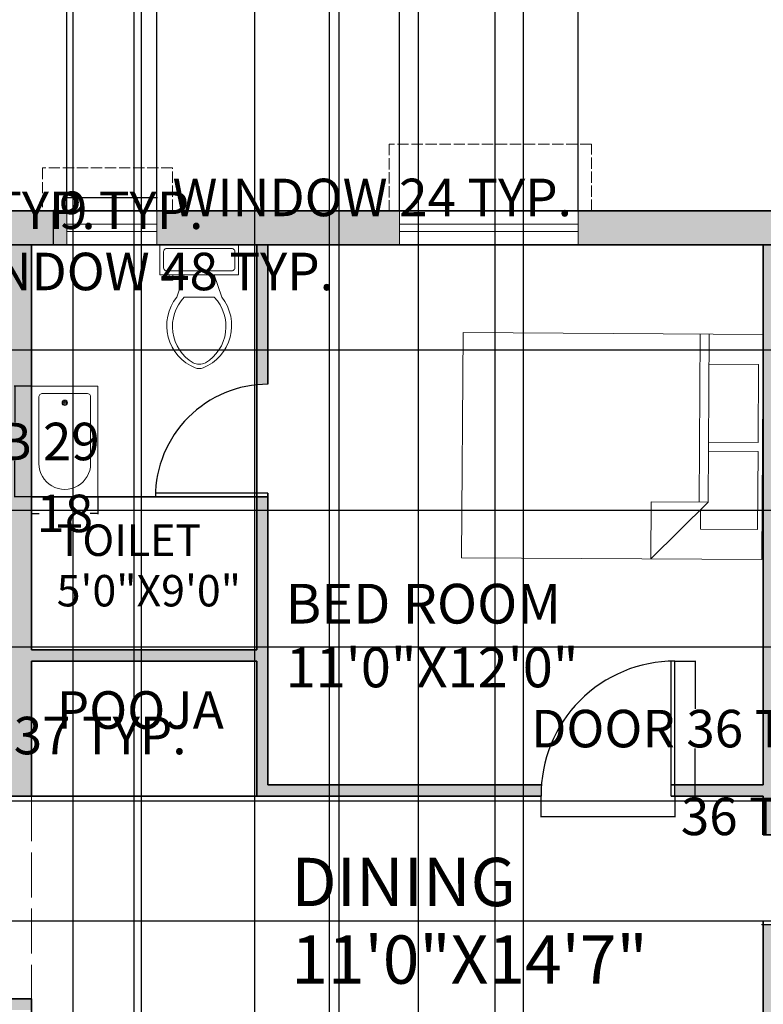
# Model space of a CAD drawing. Units: inches. Extents: x 300 to 1007, y 2 to 1069.
# Tile 5 of 12: x 568 to 766, y 271 to 533. Entities that reach past the tile are written whole.
import ezdxf

# ---------------------------------------------------------------- set-up
doc = ezdxf.new("R2010")
doc.units = ezdxf.units.IN
doc.header["$MEASUREMENT"] = 0
doc.linetypes.add('ACAD_ISO02W100', pattern=[15, 12, -3])
for name, color, linetype, lineweight in [('A-ANNO-DIMS', 2, 'Continuous', 18), ('A-AREA-IDEN', 7, 'Continuous', 18), ('A-DOOR', 3, 'Continuous', 25), ('A-FLOR-FIXT', 9, 'Continuous', 18), ('A-FURN', 8, 'Continuous', 18), ('A-GLAZ', 4, 'Continuous', 18), ('A-GLAZ-OVHD', 8, 'ACAD_ISO02W100', 13), ('A-WALL', 7, 'Continuous', 35), ('A-WALL-OVHD', 8, 'ACAD_ISO02W100', 18)]:
    doc.layers.add(name, color=color, linetype=linetype, lineweight=lineweight)
doc.layers.add('A-WALL-PATT', color=9, linetype='Continuous', lineweight=9, true_color=0xc7c8ca)
doc.styles.get("Standard").update_dxf_attribs({"font": 'arial.ttf'})
doc.dimstyles.get("Standard").update_dxf_attribs({"dimtxt": 10, "dimasz": 0.18, "dimexe": 0.18, "dimexo": 0.0625, "dimgap": 0.09, "dimtad": 0, "dimtih": 1, "dimtoh": 1, "dimdec": 0, "dimzin": 0, "dimdsep": 46, "dimlunit": 3, "dimtxsty": 'Standard', "dimcen": 0.09, "dimadec": 0, "dimazin": 0, "dimtfac": 1, "dimtdec": 0, "dimtofl": 0, "dimtmove": 0, "dimatfit": 3, "dimfxl": 1, "dimtolj": 1, "dimtzin": 0, "dimarcsym": 0})

# ---------------------------------------------------------------- blocks, each defined once
blk = doc.blocks.new('Bed - Queen')
for p, q in [((0, -80.00003), (0, 0)), ((0, 0), (59.99999, 0)), ((59.99999, 0), (59.99999, -80.00003)), ((7.99999, -1.2), (28.79998, -1.2)), ((7.99999, -14.4), (7.99999, -1.2)), ((28.79998, -1.2), (28.79998, -14.4)), ((31.19999, -1.2), (51.99999, -1.2)), ((31.19999, -14.4), (31.19999, -1.2)), ((51.99999, -1.2), (51.99999, -16.4)), ((0, -14.4), (44.8, -14.4)), ((59.99999, -29.6), (44.8, -14.4)), ((44.8, -14.4), (44.8, -29.6)), ((44.8, -16.8), (0, -16.8)), ((51.99999, -16.4), (46.79936, -16.4)), ((44.8, -29.6), (59.99999, -29.6)), ((59.99999, -80.00003), (0, -80.00003))]:
    blk.add_line(p, q)
blk = doc.blocks.new('Bath Tub - 26 x 60 in.')
for p, q in [((8, -18), (10, -18)), ((9, -17), (9, -19))]:
    blk.add_line(p, q)
blk.add_lwpolyline([(0, -36), (0, 0), (60, 0), (60, -36)], close=True)
for points in [[(6, -4), (42, -4)], [(4, -30), (4, -6)], [(42, -32), (6, -32)]]:
    blk.add_lwpolyline(points)
for radius in [1.5, 1]:
    blk.add_circle((9, -18), radius)
for centre, radius, start, end in [((5.75, -5.75), 1.77, 81.8699, 188.1301), ((42, -18), 14, 270, 90), ((5.75, -30.25), 1.77, 171.8699, 278.1301)]:
    blk.add_arc(centre, radius, start, end)
blk = doc.blocks.new('Toilet - top')
for p, q in [((9.5, -6), (9.5, -2)), ((-10, -8.5), (-8, -8.5)), ((-10, -9.5), (-10, -8.5)), ((-7, -9.5), (-10, -9.5)), ((-8, -8.5), (-8, -8)), ((-7, -8), (-7, -9.5)), ((-4, -8), (-6, -14)), ((4, -8), (6, -14)), ((4, -14), (-4, -14))]:
    blk.add_line(p, q)
blk.add_lwpolyline([(10.5, -8), (10.5, 0), (-10.5, 0), (-10.5, -8)], close=True)
for points in [[(-9.5, -2), (-9.5, -6)], [(8.5, -1), (-8.5, -1)], [(-8.5, -7), (8.5, -7)]]:
    blk.add_lwpolyline(points)
for centre, radius, start, end in [((-8.62, -1.88), 0.884, 81.8699, 188.1301), ((8.62, -1.88), 0.884, 351.8699, 98.1301), ((-8.62, -6.12), 0.884, 171.8699, 278.1301), ((8.62, -6.12), 0.884, 261.8699, 8.1301), ((3.52, -21.58), 12.17, 141.4691, 247.9714), ((4.2, -21.82), 11.33, 136.3677, 238.9468), ((-3.52, -21.58), 12.17, 292.0284, 38.5307), ((-4.2, -21.82), 11.33, 301.053, 43.6321), ((0, -27.88), 4, 245.7318, 294.2682), ((0, -29), 4, 254.8605, 285.1395)]:
    blk.add_arc(centre, radius, start, end)
blk = doc.blocks.new('WIN-47_5-8')
for p, q in [((-47.61, 0), (-47.61, 4.5)), ((-47.61, 4.5), (-47.61, -4.5)), ((0, -4.5), (0, 4.5)), ((0, 1), (-47.61, 1)), ((0, -1), (-47.61, -1))]:
    blk.add_line(p, q)
blk = doc.blocks.new('WIN-24')
for p, q in [((0, -4.5), (0, 4.5)), ((23.96, 0), (23.96, 4.5)), ((23.96, 4.5), (23.96, -4.5)), ((0, 1), (23.96, 1)), ((0, -1), (23.96, -1))]:
    blk.add_line(p, q)
blk = doc.blocks.new('WINDOW-HOOD-54')
at = {"ltscale": 0.25}
for p, q in [((0, 17.83), (-53.97, 17.83)), ((-53.97, 17.83), (-53.97, 0)), ((0, 0), (0, 17.83))]:
    blk.add_line(p, q, dxfattribs=at)
blk = doc.blocks.new('DOOR-SINGLE-30')
for p, q in [((0, 0), (30, 0)), ((0, -1), (0, 0)), ((0, -1), (30, -1))]:
    blk.add_line(p, q)
blk.add_arc((0, 0), 30, 270, 0)
blk = doc.blocks.new('DOOR-SINGLE-36')
for p, q in [((-1, 0), (-1, 36)), ((0, 0), (0, 36))]:
    blk.add_line(p, q)
blk.add_arc((0, 0.34), 35.66, 90, 180.5503)
blk = doc.blocks.new('*D35')
at = {"layer": 'A-ANNO-DIMS', "color": 0, "lineweight": -2, "transparency": 16777216}
for p, q in [((571.06, 435.66), (566.52, 435.66)), ((566.7, 435.48), (566.7, 426.11)), ((566.7, 406.35), (566.7, 415.72)), ((571.06, 406.17), (566.52, 406.17))]:
    blk.add_line(p, q, dxfattribs=at)
at = {"layer": 'A-ANNO-DIMS', "color": 0, "transparency": 16777216}
for points in [[(566.67, 435.48), (566.73, 435.48), (566.7, 435.66)], [(566.67, 406.35), (566.73, 406.35), (566.7, 406.17)]]:
    blk.add_solid(points, dxfattribs=at)
at = {"layer": 'Defpoints', "color": 0, "transparency": 16777216}
for p in [(571.12, 435.66), (566.7, 406.17), (571.12, 406.17)]:
    blk.add_point(p, dxfattribs=at)
at = {"layer": 'A-ANNO-DIMS', "color": 0, "transparency": 16777216, "insert": (566.7, 420.92), "char_height": 10, "attachment_point": 5}
blk.add_mtext('\\A1;TUB 29', dxfattribs=at)
blk = doc.blocks.new('*D36')
at = {"layer": 'A-ANNO-DIMS', "color": 0, "lineweight": -2, "transparency": 16777216}
for p, q in [((571.12, 406.11), (571.12, 401.57)), ((588.81, 406.11), (588.81, 401.57)), ((571.3, 401.75), (573.18, 401.75)), ((588.63, 401.75), (586.76, 401.75))]:
    blk.add_line(p, q, dxfattribs=at)
at = {"layer": 'A-ANNO-DIMS', "color": 0, "transparency": 16777216}
for points in [[(571.3, 401.78), (571.3, 401.72), (571.12, 401.75)], [(588.63, 401.78), (588.63, 401.72), (588.81, 401.75)]]:
    blk.add_solid(points, dxfattribs=at)
at = {"layer": 'Defpoints', "color": 0, "transparency": 16777216}
for p in [(571.12, 406.17), (588.81, 406.17), (588.81, 401.75)]:
    blk.add_point(p, dxfattribs=at)
at = {"layer": 'A-ANNO-DIMS', "color": 0, "transparency": 16777216, "insert": (579.97, 401.75), "char_height": 10, "attachment_point": 5}
blk.add_mtext('\\A1;18', dxfattribs=at)
blk = doc.blocks.new('*D52')
at = {"layer": 'A-ANNO-DIMS', "color": 0, "lineweight": -2, "transparency": 16777216}
for p, q in [((528.12, 355.06), (528.12, 342.35)), ((564.79, 355.06), (564.79, 342.35)), ((528.3, 342.53), (564.61, 342.53)), ((564.79, 342.53), (564.97, 342.53))]:
    blk.add_line(p, q, dxfattribs=at)
at = {"layer": 'A-ANNO-DIMS', "color": 0, "transparency": 16777216}
for points in [[(528.3, 342.56), (528.3, 342.5), (528.12, 342.53)], [(564.61, 342.56), (564.61, 342.5), (564.79, 342.53)]]:
    blk.add_solid(points, dxfattribs=at)
at = {"layer": 'Defpoints', "color": 0, "transparency": 16777216}
for p in [(528.12, 355.13), (564.79, 355.13), (564.79, 342.53)]:
    blk.add_point(p, dxfattribs=at)
at = {"layer": 'A-ANNO-DIMS', "color": 0, "transparency": 16777216, "insert": (589.39, 342.53), "char_height": 10, "attachment_point": 5}
blk.add_mtext('\\A1;37 TYP.', dxfattribs=at)
blk = doc.blocks.new('*D55')
at = {"layer": 'A-ANNO-DIMS', "color": 0, "lineweight": -2, "transparency": 16777216}
for p, q in [((493.48, 473.32), (493.48, 466.06)), ((541.08, 473.32), (541.08, 466.06)), ((493.66, 466.24), (540.9, 466.24)), ((541.08, 466.24), (541.26, 466.24))]:
    blk.add_line(p, q, dxfattribs=at)
at = {"layer": 'A-ANNO-DIMS', "color": 0, "transparency": 16777216}
for points in [[(493.66, 466.27), (493.66, 466.21), (493.48, 466.24)], [(540.9, 466.27), (540.9, 466.21), (541.08, 466.24)]]:
    blk.add_solid(points, dxfattribs=at)
at = {"layer": 'Defpoints', "color": 0, "transparency": 16777216}
for p in [(493.48, 473.38), (541.08, 473.38), (541.08, 466.24)]:
    blk.add_point(p, dxfattribs=at)
at = {"layer": 'A-ANNO-DIMS', "color": 0, "transparency": 16777216, "insert": (598.48, 466.24), "char_height": 10, "attachment_point": 5}
blk.add_mtext('\\A1;WINDOW 48 TYP.', dxfattribs=at)
blk = doc.blocks.new('*D56')
at = {"layer": 'A-ANNO-DIMS', "color": 0, "lineweight": -2, "transparency": 16777216}
for p, q in [((541.14, 482.38), (548.4, 482.38)), ((548.22, 482.38), (548.22, 482.56)), ((548.22, 482.56), (548.4, 482.56)), ((548.22, 473.56), (548.22, 482.2)), ((541.14, 473.38), (548.4, 473.38))]:
    blk.add_line(p, q, dxfattribs=at)
at = {"layer": 'A-ANNO-DIMS', "color": 0, "transparency": 16777216}
for points in [[(548.19, 482.2), (548.25, 482.2), (548.22, 482.38)], [(548.19, 473.56), (548.25, 473.56), (548.22, 473.38)]]:
    blk.add_solid(points, dxfattribs=at)
at = {"layer": 'Defpoints', "color": 0, "transparency": 16777216}
for p in [(541.08, 482.38), (548.22, 482.38), (541.08, 473.38)]:
    blk.add_point(p, dxfattribs=at)
at = {"layer": 'A-ANNO-DIMS', "color": 0, "transparency": 16777216, "insert": (568.95, 482.56), "char_height": 10, "attachment_point": 5}
blk.add_mtext('\\A1;9 TYP.', dxfattribs=at)
blk = doc.blocks.new('*D57')
at = {"layer": 'A-ANNO-DIMS', "color": 0, "lineweight": -2, "transparency": 16777216}
for p, q in [((580.53, 482.45), (580.53, 486.16)), ((580.71, 485.98), (604.31, 485.98)), ((604.49, 482.45), (604.49, 486.16)), ((604.49, 485.98), (604.67, 485.98))]:
    blk.add_line(p, q, dxfattribs=at)
at = {"layer": 'A-ANNO-DIMS', "color": 0, "transparency": 16777216}
for points in [[(580.71, 486.01), (580.71, 485.95), (580.53, 485.98)], [(604.31, 486.01), (604.31, 485.95), (604.49, 485.98)]]:
    blk.add_solid(points, dxfattribs=at)
at = {"layer": 'Defpoints', "color": 0, "transparency": 16777216}
for p in [(604.49, 485.98), (580.53, 482.38), (604.49, 482.38)]:
    blk.add_point(p, dxfattribs=at)
at = {"layer": 'A-ANNO-DIMS', "color": 0, "transparency": 16777216, "insert": (661.89, 485.98), "char_height": 10, "attachment_point": 5}
blk.add_mtext('\\A1;WINDOW 24 TYP.', dxfattribs=at)
blk = doc.blocks.new('*D58')
at = {"layer": 'A-ANNO-DIMS', "color": 0, "lineweight": -2, "transparency": 16777216}
for p, q in [((580.47, 482.38), (576.76, 482.38)), ((576.94, 482.38), (576.94, 482.56)), ((576.94, 482.56), (577.12, 482.56)), ((576.94, 473.56), (576.94, 482.2)), ((580.47, 473.38), (576.76, 473.38))]:
    blk.add_line(p, q, dxfattribs=at)
at = {"layer": 'A-ANNO-DIMS', "color": 0, "transparency": 16777216}
for points in [[(576.91, 482.2), (576.97, 482.2), (576.94, 482.38)], [(576.91, 473.56), (576.97, 473.56), (576.94, 473.38)]]:
    blk.add_solid(points, dxfattribs=at)
at = {"layer": 'Defpoints', "color": 0, "transparency": 16777216}
for p in [(576.94, 482.38), (580.53, 482.38), (580.53, 473.38)]:
    blk.add_point(p, dxfattribs=at)
at = {"layer": 'A-ANNO-DIMS', "color": 0, "transparency": 16777216, "insert": (597.66, 482.56), "char_height": 10, "attachment_point": 5}
blk.add_mtext('\\A1;9 TYP.', dxfattribs=at)
blk = doc.blocks.new('*D65')
at = {"layer": 'A-ANNO-DIMS', "color": 0, "lineweight": -2, "transparency": 16777216}
for p, q in [((742.62, 362.38), (748.14, 362.38)), ((747.96, 362.2), (747.96, 349.65)), ((747.96, 326.56), (747.96, 339.12)), ((742.62, 326.38), (748.14, 326.38))]:
    blk.add_line(p, q, dxfattribs=at)
at = {"layer": 'A-ANNO-DIMS', "color": 0, "transparency": 16777216}
for points in [[(747.93, 362.2), (747.99, 362.2), (747.96, 362.38)], [(747.93, 326.56), (747.99, 326.56), (747.96, 326.38)]]:
    blk.add_solid(points, dxfattribs=at)
at = {"layer": 'Defpoints', "color": 0, "transparency": 16777216}
for p in [(742.56, 362.38), (747.96, 362.38), (742.56, 326.38)]:
    blk.add_point(p, dxfattribs=at)
at = {"layer": 'A-ANNO-DIMS', "color": 0, "transparency": 16777216, "insert": (747.96, 344.38), "char_height": 10, "attachment_point": 5}
blk.add_mtext('\\A1;DOOR 36 TYP.', dxfattribs=at)
blk = doc.blocks.new('*D66')
at = {"layer": 'A-ANNO-DIMS', "color": 0, "lineweight": -2, "transparency": 16777216}
for p, q in [((706.81, 326.32), (706.81, 320.8)), ((742.56, 326.32), (742.56, 320.8)), ((706.99, 320.98), (742.38, 320.98)), ((742.56, 320.98), (742.74, 320.98))]:
    blk.add_line(p, q, dxfattribs=at)
at = {"layer": 'A-ANNO-DIMS', "color": 0, "transparency": 16777216}
for points in [[(706.99, 321.01), (706.99, 320.95), (706.81, 320.98)], [(742.38, 321.01), (742.38, 320.95), (742.56, 320.98)]]:
    blk.add_solid(points, dxfattribs=at)
at = {"layer": 'Defpoints', "color": 0, "transparency": 16777216}
for p in [(706.81, 326.38), (742.56, 326.38), (742.56, 320.98)]:
    blk.add_point(p, dxfattribs=at)
at = {"layer": 'A-ANNO-DIMS', "color": 0, "transparency": 16777216, "insert": (767.16, 320.98), "char_height": 10, "attachment_point": 5}
blk.add_mtext('\\A1;36 TYP.', dxfattribs=at)
blk = doc.blocks.new('*D89')
at = {"layer": 'A-ANNO-DIMS', "color": 0, "lineweight": -2, "transparency": 16777216}
for p, q in [((544.6, 83.45), (544.6, 1063.03)), ((544.78, 1062.85), (554.56, 1062.85)), ((598.25, 1062.85), (588.48, 1062.85)), ((598.43, 83.45), (598.43, 1063.03))]:
    blk.add_line(p, q, dxfattribs=at)
at = {"layer": 'A-ANNO-DIMS', "color": 0, "transparency": 16777216}
for points in [[(544.78, 1062.88), (544.78, 1062.82), (544.6, 1062.85)], [(598.25, 1062.88), (598.25, 1062.82), (598.43, 1062.85)]]:
    blk.add_solid(points, dxfattribs=at)
at = {"layer": 'Defpoints', "color": 0, "transparency": 16777216}
for p in [(598.43, 1062.85), (544.6, 83.38), (598.43, 83.38)]:
    blk.add_point(p, dxfattribs=at)
at = {"layer": 'A-ANNO-DIMS', "color": 0, "transparency": 16777216, "insert": (571.52, 1062.85), "char_height": 10, "attachment_point": 5}
blk.add_mtext('\\A1;53.83', dxfattribs=at)
blk = doc.blocks.new('*D91')
at = {"layer": 'A-ANNO-DIMS', "color": 0, "lineweight": -2, "transparency": 16777216}
for p, q in [((429.18, 325.09), (974.48, 325.09)), ((974.3, 324.91), (974.3, 290.23)), ((974.3, 245.16), (974.3, 279.84)), ((429.18, 244.98), (974.48, 244.98))]:
    blk.add_line(p, q, dxfattribs=at)
at = {"layer": 'A-ANNO-DIMS', "color": 0, "transparency": 16777216}
for points in [[(974.27, 324.91), (974.33, 324.91), (974.3, 325.09)], [(974.27, 245.16), (974.33, 245.16), (974.3, 244.98)]]:
    blk.add_solid(points, dxfattribs=at)
at = {"layer": 'Defpoints', "color": 0, "transparency": 16777216}
for p in [(429.12, 325.09), (974.3, 325.09), (429.12, 244.98)]:
    blk.add_point(p, dxfattribs=at)
at = {"layer": 'A-ANNO-DIMS', "color": 0, "transparency": 16777216, "insert": (974.3, 285.04), "char_height": 10, "attachment_point": 5}
blk.add_mtext('\\A1;80.11', dxfattribs=at)
blk = doc.blocks.new('*D92')
at = {"layer": 'A-ANNO-DIMS', "color": 0, "lineweight": -2, "transparency": 16777216}
for p, q in [((429.18, 473.38), (974.48, 473.38)), ((974.3, 473.2), (974.3, 464.54)), ((974.3, 445.49), (974.3, 454.15)), ((429.18, 445.31), (974.48, 445.31))]:
    blk.add_line(p, q, dxfattribs=at)
at = {"layer": 'A-ANNO-DIMS', "color": 0, "transparency": 16777216}
for points in [[(974.27, 473.2), (974.33, 473.2), (974.3, 473.38)], [(974.27, 445.49), (974.33, 445.49), (974.3, 445.31)]]:
    blk.add_solid(points, dxfattribs=at)
at = {"layer": 'Defpoints', "color": 0, "transparency": 16777216}
for p in [(429.12, 473.38), (429.12, 445.31), (974.3, 445.31)]:
    blk.add_point(p, dxfattribs=at)
at = {"layer": 'A-ANNO-DIMS', "color": 0, "transparency": 16777216, "insert": (974.3, 459.35), "char_height": 10, "attachment_point": 5}
blk.add_mtext('\\A1;28.07', dxfattribs=at)
blk = doc.blocks.new('*D95')
at = {"layer": 'A-ANNO-DIMS', "color": 0, "lineweight": -2, "transparency": 16777216}
for p, q in [((901.06, 473.38), (354.19, 473.38)), ((354.37, 473.2), (354.37, 443.16)), ((354.37, 402.72), (354.37, 432.77)), ((901.06, 402.54), (354.19, 402.54))]:
    blk.add_line(p, q, dxfattribs=at)
at = {"layer": 'A-ANNO-DIMS', "color": 0, "transparency": 16777216}
for points in [[(354.34, 473.2), (354.4, 473.2), (354.37, 473.38)], [(354.34, 402.72), (354.4, 402.72), (354.37, 402.54)]]:
    blk.add_solid(points, dxfattribs=at)
at = {"layer": 'Defpoints', "color": 0, "transparency": 16777216}
for p in [(354.37, 473.38), (901.12, 473.38), (901.12, 402.54)]:
    blk.add_point(p, dxfattribs=at)
at = {"layer": 'A-ANNO-DIMS', "color": 0, "transparency": 16777216, "insert": (354.37, 437.96), "char_height": 10, "attachment_point": 5}
blk.add_mtext('\\A1;70.85', dxfattribs=at)
blk = doc.blocks.new('*D96')
at = {"layer": 'A-ANNO-DIMS', "color": 0, "lineweight": -2, "transparency": 16777216}
for p, q in [((901.06, 366.1), (354.19, 366.1)), ((354.37, 365.92), (354.37, 334.77)), ((354.37, 293.21), (354.37, 324.37)), ((901.06, 293.03), (354.19, 293.03))]:
    blk.add_line(p, q, dxfattribs=at)
at = {"layer": 'A-ANNO-DIMS', "color": 0, "transparency": 16777216}
for points in [[(354.34, 365.92), (354.4, 365.92), (354.37, 366.1)], [(354.34, 293.21), (354.4, 293.21), (354.37, 293.03)]]:
    blk.add_solid(points, dxfattribs=at)
at = {"layer": 'Defpoints', "color": 0, "transparency": 16777216}
for p in [(354.37, 366.1), (901.12, 366.1), (901.12, 293.03)]:
    blk.add_point(p, dxfattribs=at)
at = {"layer": 'A-ANNO-DIMS', "color": 0, "transparency": 16777216, "insert": (354.37, 329.57), "char_height": 10, "attachment_point": 5}
blk.add_mtext('\\A1;73.07', dxfattribs=at)
blk = doc.blocks.new('*D98')
at = {"layer": 'A-ANNO-DIMS', "color": 0, "lineweight": -2, "transparency": 16777216}
for p, q in [((541.08, 482.45), (541.08, 1063.03)), ((541.26, 1062.85), (543.81, 1062.85)), ((580.35, 1062.85), (577.8, 1062.85)), ((580.53, 482.45), (580.53, 1063.03))]:
    blk.add_line(p, q, dxfattribs=at)
at = {"layer": 'A-ANNO-DIMS', "color": 0, "transparency": 16777216}
for points in [[(541.26, 1062.88), (541.26, 1062.82), (541.08, 1062.85)], [(580.35, 1062.88), (580.35, 1062.82), (580.53, 1062.85)]]:
    blk.add_solid(points, dxfattribs=at)
at = {"layer": 'Defpoints', "color": 0, "transparency": 16777216}
for p in [(580.53, 1062.85), (541.08, 482.38), (580.53, 482.38)]:
    blk.add_point(p, dxfattribs=at)
at = {"layer": 'A-ANNO-DIMS', "color": 0, "transparency": 16777216, "insert": (560.81, 1062.85), "char_height": 10, "attachment_point": 5}
blk.add_mtext('\\A1;39.45', dxfattribs=at)
blk = doc.blocks.new('*D99')
at = {"layer": 'A-ANNO-DIMS', "color": 0, "lineweight": -2, "transparency": 16777216}
for p, q in [((604.49, 482.45), (604.49, 1063.03)), ((604.67, 1062.85), (619.83, 1062.85)), ((668.97, 1062.85), (653.8, 1062.85)), ((669.15, 482.45), (669.15, 1063.03))]:
    blk.add_line(p, q, dxfattribs=at)
at = {"layer": 'A-ANNO-DIMS', "color": 0, "transparency": 16777216}
for points in [[(604.67, 1062.88), (604.67, 1062.82), (604.49, 1062.85)], [(668.97, 1062.88), (668.97, 1062.82), (669.15, 1062.85)]]:
    blk.add_solid(points, dxfattribs=at)
at = {"layer": 'Defpoints', "color": 0, "transparency": 16777216}
for p in [(669.15, 1062.85), (604.49, 482.38), (669.15, 482.38)]:
    blk.add_point(p, dxfattribs=at)
at = {"layer": 'A-ANNO-DIMS', "color": 0, "transparency": 16777216, "insert": (636.82, 1062.85), "char_height": 10, "attachment_point": 5}
blk.add_mtext('\\A1;64.66', dxfattribs=at)
blk = doc.blocks.new('*D100')
at = {"layer": 'A-ANNO-DIMS', "color": 0, "lineweight": -2, "transparency": 16777216}
for p, q in [((716.78, 482.45), (716.78, 1063.03)), ((716.96, 1062.85), (734.53, 1062.85)), ((786.04, 1062.85), (768.47, 1062.85)), ((786.22, 482.45), (786.22, 1063.03))]:
    blk.add_line(p, q, dxfattribs=at)
at = {"layer": 'A-ANNO-DIMS', "color": 0, "transparency": 16777216}
for points in [[(716.96, 1062.88), (716.96, 1062.82), (716.78, 1062.85)], [(786.04, 1062.88), (786.04, 1062.82), (786.22, 1062.85)]]:
    blk.add_solid(points, dxfattribs=at)
at = {"layer": 'Defpoints', "color": 0, "transparency": 16777216}
for p in [(786.22, 1062.85), (716.78, 482.38), (786.22, 482.38)]:
    blk.add_point(p, dxfattribs=at)
at = {"layer": 'A-ANNO-DIMS', "color": 0, "transparency": 16777216, "insert": (751.5, 1062.85), "char_height": 10, "attachment_point": 5}
blk.add_mtext('\\A1;69.44', dxfattribs=at)
blk = doc.blocks.new('*D102')
at = {"layer": 'A-ANNO-DIMS', "color": 0, "lineweight": -2, "transparency": 16777216}
for p, q in [((600.34, 609.38), (600.34, 8.45)), ((652.99, 609.38), (652.99, 8.45)), ((600.52, 8.63), (609.71, 8.63)), ((652.81, 8.63), (643.62, 8.63))]:
    blk.add_line(p, q, dxfattribs=at)
at = {"layer": 'A-ANNO-DIMS', "color": 0, "transparency": 16777216}
for points in [[(600.52, 8.66), (600.52, 8.6), (600.34, 8.63)], [(652.81, 8.66), (652.81, 8.6), (652.99, 8.63)]]:
    blk.add_solid(points, dxfattribs=at)
at = {"layer": 'Defpoints', "color": 0, "transparency": 16777216}
for p in [(600.34, 609.45), (652.99, 609.45), (652.99, 8.63)]:
    blk.add_point(p, dxfattribs=at)
at = {"layer": 'A-ANNO-DIMS', "color": 0, "transparency": 16777216, "insert": (626.66, 8.63), "char_height": 10, "attachment_point": 5}
blk.add_mtext('\\A1;52.66', dxfattribs=at)
blk = doc.blocks.new('*D103')
at = {"layer": 'A-ANNO-DIMS', "color": 0, "lineweight": -2, "transparency": 16777216}
for p, q in [((652.99, 609.38), (652.99, 8.45)), ((674.16, 609.38), (674.16, 8.45)), ((653.17, 8.63), (673.98, 8.63)), ((674.16, 8.63), (674.34, 8.63))]:
    blk.add_line(p, q, dxfattribs=at)
at = {"layer": 'A-ANNO-DIMS', "color": 0, "transparency": 16777216}
for points in [[(653.17, 8.66), (653.17, 8.6), (652.99, 8.63)], [(673.98, 8.66), (673.98, 8.6), (674.16, 8.63)]]:
    blk.add_solid(points, dxfattribs=at)
at = {"layer": 'Defpoints', "color": 0, "transparency": 16777216}
for p in [(652.99, 609.45), (674.16, 609.45), (674.16, 8.63)]:
    blk.add_point(p, dxfattribs=at)
at = {"layer": 'A-ANNO-DIMS', "color": 0, "transparency": 16777216, "insert": (695.25, 8.63), "char_height": 10, "attachment_point": 5}
blk.add_mtext('\\A1;21.164', dxfattribs=at)
blk = doc.blocks.new('*D104')
at = {"layer": 'A-ANNO-DIMS', "color": 0, "lineweight": -2, "transparency": 16777216}
for p, q in [((674.16, 609.38), (674.16, 8.45)), ((694.58, 609.38), (694.58, 8.45)), ((674.34, 8.63), (694.4, 8.63)), ((694.58, 8.63), (694.76, 8.63))]:
    blk.add_line(p, q, dxfattribs=at)
at = {"layer": 'A-ANNO-DIMS', "color": 0, "transparency": 16777216}
for points in [[(674.34, 8.66), (674.34, 8.6), (674.16, 8.63)], [(694.4, 8.66), (694.4, 8.6), (694.58, 8.63)]]:
    blk.add_solid(points, dxfattribs=at)
at = {"layer": 'Defpoints', "color": 0, "transparency": 16777216}
for p in [(674.16, 609.45), (694.58, 609.45), (694.58, 8.63)]:
    blk.add_point(p, dxfattribs=at)
at = {"layer": 'A-ANNO-DIMS', "color": 0, "transparency": 16777216, "insert": (711.75, 8.63), "char_height": 10, "attachment_point": 5}
blk.add_mtext('\\A1;20.42', dxfattribs=at)
blk = doc.blocks.new('*D106')
at = {"layer": 'A-ANNO-DIMS', "color": 0, "lineweight": -2, "transparency": 16777216}
for p, q in [((582.11, 990.38), (582.11, 8.45)), ((630.49, 990.38), (630.49, 8.45)), ((582.29, 8.63), (589.12, 8.63)), ((630.31, 8.63), (623.47, 8.63))]:
    blk.add_line(p, q, dxfattribs=at)
at = {"layer": 'A-ANNO-DIMS', "color": 0, "transparency": 16777216}
for points in [[(582.29, 8.66), (582.29, 8.6), (582.11, 8.63)], [(630.31, 8.66), (630.31, 8.6), (630.49, 8.63)]]:
    blk.add_solid(points, dxfattribs=at)
at = {"layer": 'Defpoints', "color": 0, "transparency": 16777216}
for p in [(582.11, 990.45), (630.49, 990.45), (630.49, 8.63)]:
    blk.add_point(p, dxfattribs=at)
at = {"layer": 'A-ANNO-DIMS', "color": 0, "transparency": 16777216, "insert": (606.3, 8.63), "char_height": 10, "attachment_point": 5}
blk.add_mtext('\\A1;48.38', dxfattribs=at)
blk = doc.blocks.new('*D107')
at = {"layer": 'A-ANNO-DIMS', "color": 0, "lineweight": -2, "transparency": 16777216}
for p, q in [((630.49, 990.38), (630.49, 8.45)), ((650.47, 990.38), (650.47, 8.45)), ((630.67, 8.63), (650.29, 8.63)), ((650.47, 8.63), (650.65, 8.63))]:
    blk.add_line(p, q, dxfattribs=at)
at = {"layer": 'A-ANNO-DIMS', "color": 0, "transparency": 16777216}
for points in [[(630.67, 8.66), (630.67, 8.6), (630.49, 8.63)], [(650.29, 8.66), (650.29, 8.6), (650.47, 8.63)]]:
    blk.add_solid(points, dxfattribs=at)
at = {"layer": 'Defpoints', "color": 0, "transparency": 16777216}
for p in [(630.49, 990.45), (650.47, 990.45), (650.47, 8.63)]:
    blk.add_point(p, dxfattribs=at)
at = {"layer": 'A-ANNO-DIMS', "color": 0, "transparency": 16777216, "insert": (667.15, 8.63), "char_height": 10, "attachment_point": 5}
blk.add_mtext('\\A1;19.98', dxfattribs=at)
blk = doc.blocks.new('*D108')
at = {"layer": 'A-ANNO-DIMS', "color": 0, "lineweight": -2, "transparency": 16777216}
for p, q in [((650.47, 990.38), (650.47, 8.45)), ((702.09, 990.38), (702.09, 8.45)), ((650.65, 8.63), (659.37, 8.63)), ((701.91, 8.63), (693.19, 8.63))]:
    blk.add_line(p, q, dxfattribs=at)
at = {"layer": 'A-ANNO-DIMS', "color": 0, "transparency": 16777216}
for points in [[(650.65, 8.66), (650.65, 8.6), (650.47, 8.63)], [(701.91, 8.66), (701.91, 8.6), (702.09, 8.63)]]:
    blk.add_solid(points, dxfattribs=at)
at = {"layer": 'Defpoints', "color": 0, "transparency": 16777216}
for p in [(650.47, 990.45), (702.09, 990.45), (702.09, 8.63)]:
    blk.add_point(p, dxfattribs=at)
at = {"layer": 'A-ANNO-DIMS', "color": 0, "transparency": 16777216, "insert": (676.28, 8.63), "char_height": 10, "attachment_point": 5}
blk.add_mtext('\\A1;51.62', dxfattribs=at)
blk = doc.blocks.new('*D119')
at = {"layer": 'A-ANNO-DIMS', "color": 0, "lineweight": -2, "transparency": 16777216}
for p, q in [((793.02, 319.02), (782.94, 309.07)), ((793.2, 319.02), (793.02, 319.02)), ((765.69, 292.16), (765.87, 292.16)), ((765.78, 292.07), (765.78, 292.25))]:
    blk.add_line(p, q, dxfattribs=at)
at = {"layer": 'A-ANNO-DIMS', "color": 0, "transparency": 16777216}
blk.add_solid([(782.92, 309.09), (782.96, 309.05), (782.81, 308.94)], dxfattribs=at)
at = {"layer": 'Defpoints', "color": 0, "transparency": 16777216}
for p in [(782.81, 308.94), (765.78, 292.16)]:
    blk.add_point(p, dxfattribs=at)
at = {"layer": 'A-ANNO-DIMS', "color": 0, "transparency": 16777216, "insert": (813.99, 319.02), "char_height": 10, "attachment_point": 5}
blk.add_mtext('\\A1;R23.91', dxfattribs=at)

msp = doc.modelspace()

# ---------------------------------------------------------------- hatches: boundary and pattern name
at = {"layer": 'A-WALL-PATT'}
h = msp.add_hatch(color=256, dxfattribs=at)
h.dxf.hatch_style = 1
h.paths.add_polyline_path([(546.104, 999.4468), (478.8267, 999.4468), (478.8267, 869.2798, -0.06322715), (487.8267, 868.1328), (487.8267, 990.4468), (546.104, 990.4468)])
h.paths.add_polyline_path([(630.4852, 999.4468), (582.106, 999.4468), (582.106, 990.4468), (613.8267, 990.4468), (613.8267, 867.4468), (622.8267, 867.4468), (622.8267, 990.4468), (630.4852, 990.4468)])
h.paths.add_polyline_path([(702.0883, 999.4468), (650.4653, 999.4468), (650.4653, 990.4468), (682.8267, 990.4468), (682.8267, 960.0824, -0.02530575), (685.8267, 960.0478), (685.8267, 990.4468), (702.0883, 990.4468)])
h.paths.add_polyline_path([(850.8267, 999.4468), (737.5888, 999.4468), (737.5888, 990.4468), (841.8267, 990.4468), (841.8267, 950.5685), (850.8267, 950.5685)])
h.paths.add_polyline_path([(685.8267, 930.4465), (682.8267, 930.4465), (682.8267, 888.4468), (682.8267, 867.4468), (685.8267, 867.4468), (697.4169, 867.4468), (697.4169, 870.4468), (685.8267, 870.4468), (685.8267, 888.4468)])
h.paths.add_polyline_path([(682.8267, 931.4465), (654.3436, 931.4465, 0.00843109), (654.3267, 930.4465), (682.8267, 930.4465)])
h.paths.add_polyline_path([(685.8267, 931.4465), (682.8267, 931.4465), (682.8267, 930.4465), (685.8267, 930.4465)])
h.paths.add_polyline_path([(682.8267, 888.4468), (622.8267, 888.4468), (622.8267, 885.4468), (682.8267, 885.4468)])
h.paths.add_polyline_path([(850.8267, 870.4468), (850.8267, 914.7851), (841.8267, 914.7851), (841.8267, 870.4468), (732.7101, 870.4468, -0.02120595), (732.8267, 867.4468), (779.8267, 867.4468), (779.8267, 749.4468), (782.8267, 749.4468), (788.8267, 749.4468), (788.8267, 861.4468), (841.8267, 861.4468), (841.8267, 749.4468), (850.8267, 749.4468)])
h.paths.add_polyline_path([(622.8267, 810.4468), (487.8267, 810.4468), (487.8267, 833.2626), (478.8267, 833.2626), (478.8267, 609.4468), (478.8267, 482.3847), (487.8267, 482.3847), (487.8267, 801.4468), (620.8267, 801.4468), (622.8267, 801.4468)])
h.paths.add_polyline_path([(680.8267, 729.4468), (620.8267, 729.4468), (620.8267, 765.8246, -0.02111352), (617.8267, 766.0562), (617.8267, 698.7303), (620.8267, 698.7303), (620.8267, 726.4468), (680.8267, 726.4468)])
h.paths.add_polyline_path([(620.8267, 668.8122, -0.02498293), (617.8267, 668.6448), (617.8267, 618.4468), (600.3357, 618.4468), (600.3357, 609.4468), (652.9929, 609.4468), (652.9929, 618.4468), (620.8267, 618.4468)])
h.paths.add_polyline_path([(552.3393, 618.4468), (487.8267, 618.4468), (487.8267, 609.4468), (552.3393, 609.4468)], flags=17)
h.paths.add_polyline_path([(694.5763, 618.4468), (683.8267, 618.4468), (683.8267, 726.4468), (683.8267, 749.4468), (680.8267, 749.4468), (680.8267, 740.4468), (680.8267, 726.4468), (680.8267, 618.4468), (674.1573, 618.4468), (674.1573, 609.4468), (680.8267, 609.4468), (694.5763, 609.4468)])
h.paths.add_polyline_path([(850.8267, 642.8902), (841.8267, 642.8902), (841.8267, 618.4468), (782.8267, 618.4468), (782.8267, 708.0513, -0.02308839), (779.8267, 707.9092), (779.8267, 618.4468), (730.1068, 618.4468), (730.1068, 609.4468), (779.8267, 609.4468), (841.8267, 609.4468), (841.8267, 482.3847), (850.8267, 482.3847)])
h.paths.add_polyline_path([(850.8267, 749.4468), (841.8267, 749.4468), (841.8267, 705.9119), (850.8267, 705.9119)])
h.paths.add_polyline_path([(841.8267, 749.4468), (782.8267, 749.4468), (779.8267, 749.4468), (761.9959, 749.4468), (761.9959, 740.4468), (779.8267, 740.4468), (812.3267, 740.4468), (841.8267, 740.4468)])
h.paths.add_polyline_path([(669.1457, 482.3847), (604.489, 482.3847), (604.489, 473.3847), (631.1217, 473.3847), (631.1217, 436.0244, -0.02504709), (634.1217, 436.1748), (634.1217, 436.4367), (634.1217, 473.3847), (669.1457, 473.3847)], flags=17)
h.paths.add_polyline_path([(580.5305, 482.3847), (571.1217, 482.3847), (541.0813, 482.3847), (541.0813, 473.3847), (562.1217, 473.3847), (562.1217, 326.3847), (571.1217, 326.3847), (571.1217, 362.3847), (631.1217, 362.3847), (631.1217, 326.3847), (706.9024, 326.3847, -0.02105388), (706.9999, 329.3847), (634.1217, 329.3847), (634.1217, 365.3847), (634.1217, 406.1748), (631.1217, 406.1748), (631.1217, 365.3847), (571.1217, 365.3847), (571.1217, 473.3847), (580.5305, 473.3847)])
h.paths.add_polyline_path([(493.4756, 482.3847), (420.1217, 482.3847), (420.1217, 445.3134), (429.1217, 445.3134), (429.1217, 473.3847), (493.4756, 473.3847)])
h.paths.add_polyline_path([(786.2236, 482.3847), (716.7793, 482.3847), (716.7793, 473.3847), (766.1217, 473.3847), (766.1217, 329.3847), (742.5583, 329.3847), (742.5583, 326.3847), (766.1217, 326.3847), (766.1217, 316.0647), (769.1217, 316.0647), (769.1217, 326.3847), (769.1217, 473.3847), (786.2236, 473.3847)])
h.paths.add_polyline_path([(910.1217, 482.3847), (822.7166, 482.3847), (822.7166, 473.3847), (901.1217, 473.3847), (901.1217, 402.5393), (910.1217, 402.5393)])
h.paths.add_polyline_path([(910.1217, 366.1034), (901.1217, 366.1034), (901.1217, 329.3847), (814.1217, 329.3847), (814.1217, 312.5176), (817.1217, 312.5176), (817.1217, 326.3847), (901.1217, 326.3847), (901.1217, 293.0319), (910.1217, 293.0319), (910.1217, 326.3847)])
h.paths.add_polyline_path([(910.1217, 268.9355), (901.1217, 268.9355), (901.1217, 254.3847), (817.1217, 254.3847), (817.1217, 290.5411, -0.03396715), (814.1217, 290.3847), (814.1217, 254.3847), (775.1217, 254.3847), (775.1217, 281.5164), (769.1217, 281.5164), (769.1217, 292.1577), (766.1217, 292.1577), (766.1217, 254.3847), (766.1217, 220.1938), (775.5079, 220.1938), (775.5079, 251.3847), (817.1217, 251.3847), (901.1217, 251.3847), (901.1217, 152.3847), (819.0246, 152.3847, -0.02493798), (818.9117, 149.3847), (901.1217, 149.3847), (901.1217, 92.3847), (901.1217, 83.3847), (874.3528, 83.3847), (874.3528, 74.3847), (910.1217, 74.3847), (910.1217, 92.3847), (910.1217, 149.3847)])
h.paths.add_polyline_path([(429.1217, 325.0924), (420.1217, 325.0924), (420.1217, 263.3847), (420.1217, 244.9834), (429.1217, 244.9834), (429.1217, 269.3847), (571.1217, 269.3847), (571.1217, 272.3847), (562.1217, 272.3847), (429.1217, 272.3847)])
h.paths.add_polyline_path([(429.1217, 208.998), (420.1217, 208.998), (420.1217, 74.3847), (496.7704, 74.3847), (496.7704, 83.3847), (429.1217, 83.3847)])
h.paths.add_polyline_path([(598.4322, 83.3847), (571.1217, 83.3847), (571.1217, 122.1171), (562.1217, 122.1171), (562.1217, 83.3847), (544.6031, 83.3847), (544.6031, 74.3847), (598.4322, 74.3847)])
h.paths.add_polyline_path([(797.0822, 83.3847), (769.1217, 83.3847), (769.1217, 149.3847), (788.9123, 149.3847), (788.9123, 152.3847), (769.1217, 152.3847), (769.1217, 178.0167), (766.1217, 178.0167), (766.1217, 152.3847), (735.3598, 152.3847), (735.3598, 143.3847), (766.1217, 143.3847), (766.1217, 83.3847), (634.1217, 83.3847), (634.1217, 143.3847), (659.7326, 143.3847), (659.7326, 152.3847), (634.1217, 152.3847), (634.1217, 194.3847), (571.1217, 194.3847), (571.1217, 233.7289, -0.06379947), (562.1217, 234.7942), (562.1217, 163.4485), (567.7403, 163.4485), (567.7403, 152.3847), (571.1217, 152.3847), (571.1217, 191.3847), (631.1217, 191.3847), (631.1217, 83.3847), (621.979, 83.3847), (621.979, 74.3847), (631.1217, 74.3847), (797.0822, 74.3847)])

# ---------------------------------------------------------------- linework, layer by layer
at = {"layer": 'A-DOOR'}
for p, q in [((634.1217, 406.1748), (634.1217, 407.1748)), ((634.1217, 406.1748), (604.1587, 406.1748)), ((742.5583, 326.3847), (742.5583, 329.3847)), ((742.5583, 326.3847), (741.5583, 326.3847)), ((766.1217, 293.1577), (789.6933, 293.1577)), ((766.1217, 292.1577), (789.6933, 292.1577))]:
    msp.add_line(p, q, dxfattribs=at)
at = {"layer": 'A-GLAZ-OVHD', "ltscale": 0.25}
for p, q in [((608.6839, 493.8408), (574.0095, 493.8408)), ((574.0095, 493.8408), (574.0095, 482.3847)), ((608.6839, 482.3847), (608.6839, 493.8408))]:
    msp.add_line(p, q, dxfattribs=at)
at = {"layer": 'A-WALL'}
for p, q in [((571.1217, 482.3847), (910.1217, 482.3847)), ((571.1217, 473.3847), (631.1217, 473.3847)), ((631.1217, 473.3847), (631.1217, 365.3847)), ((634.1217, 473.3847), (634.1217, 436.1748)), ((634.1217, 473.3847), (766.1217, 473.3847)), ((766.1217, 473.3847), (766.1217, 329.3847)), ((634.1217, 436.1748), (634.1217, 436.4367)), ((634.1217, 407.1748), (634.1217, 365.3847)), ((634.1217, 406.1748), (571.1217, 406.1748)), ((631.1217, 365.3847), (571.1217, 365.3847)), ((634.1217, 329.3847), (634.1217, 365.3847)), ((631.1217, 362.3847), (571.1217, 362.3847)), ((631.1217, 326.3847), (631.1217, 362.3847)), ((706.9999, 329.3847), (634.1217, 329.3847)), ((766.1217, 329.3847), (741.5583, 329.3847)), ((631.1217, 326.3847), (562.1217, 326.3847)), ((706.9024, 326.3847), (631.1217, 326.3847)), ((706.9024, 326.3847), (631.1217, 326.3847)), ((766.1217, 326.3847), (741.5583, 326.3847)), ((766.1217, 326.3847), (741.5583, 326.3847)), ((766.1217, 326.3847), (766.1217, 316.0647)), ((769.1217, 316.0647), (766.1217, 316.0647)), ((766.1217, 293.1577), (766.1217, 254.3847)), ((562.1217, 272.3847), (571.1217, 272.3847))]:
    msp.add_line(p, q, dxfattribs=at)
for points in [[(571.1217, 482.3847), (420.1217, 482.3847), (420.1217, 263.3847)], [(571.1217, 365.3847), (571.1217, 473.3847)], [(571.1217, 326.3847), (571.1217, 362.3847)], [(571.1217, 268.3847), (571.1217, 272.3847)]]:
    msp.add_lwpolyline(points, dxfattribs=at)
at = {"layer": 'A-WALL-OVHD'}
msp.add_line((571.1217, 326.3847), (571.1217, 272.3847), dxfattribs=at)

# ---------------------------------------------------------------- block references
at = {"layer": 'A-DOOR', "rotation": 180}
msp.add_blockref('DOOR-SINGLE-30', (634.1217, 406.1748), dxfattribs=at)
at = {"layer": 'A-DOOR'}
msp.add_blockref('DOOR-SINGLE-36', (742.5583, 326.3847), dxfattribs=at)
at = {"layer": 'A-FLOR-FIXT'}
msp.add_blockref('Toilet - top', (615.7964, 473.3847), dxfattribs=at)
at = {"layer": 'A-FLOR-FIXT', "xscale": 0.4914410093804691, "yscale": 0.4914410093804691, "zscale": 0.4914410093804691, "rotation": 270}
msp.add_blockref('Bath Tub - 26 x 60 in.', (588.8136, 435.6613), dxfattribs=at)
at = {"layer": 'A-FURN', "rotation": 269.6247822007257}
msp.add_blockref('Bed - Queen', (766.1217, 449.4157), dxfattribs=at)
at = {"layer": 'A-GLAZ'}
msp.add_blockref('WIN-24', (580.5305, 477.8847), dxfattribs=at)
at = {"layer": 'A-GLAZ', "extrusion": (0, 0, -1), "xscale": 1.000586652537538, "zscale": -1}
msp.add_blockref('WIN-47_5-8', (-669.1457, 477.8847), dxfattribs=at)
at = {"layer": 'A-GLAZ-OVHD'}
msp.add_blockref('WINDOW-HOOD-54', (720.3593, 482.3847), dxfattribs=at)

# ---------------------------------------------------------------- texts
at = {"layer": 'A-AREA-IDEN'}
for s, height, p in [('TOILET', 8.3808, (577.8132, 390.4146)), ('5\'0"X9\'0"', 8.3808, (577.8132, 376.9516)), ('BED ROOM', 10.58137, (638.824, 372.3902)), ('11\'0"X12\'0"', 10.581373, (638.824, 355.3921)), ('POOJA', 10.0199, (577.8132, 344.3228)), ('DINING', 12.87594, (640.3425, 297.0563)), ('11\'0"X14\'7"', 12.875935, (640.3425, 276.3722))]:
    msp.add_text(s, height=height, dxfattribs=at).set_placement(p)

# ---------------------------------------------------------------- dimensions: what is measured, and where the dimension line sits
at = {"layer": 'A-ANNO-DIMS'}
for base, p1, p2, override, picture, middle in [((580.5305, 1062.8469), (541.0813, 482.3847), (580.5305, 482.3847), {"dimdec": 2, "dimlfac": 1, "dimrnd": 0, "dimzin": 0, "dimdsep": 46, "dimlunit": 2}, '*D98', (560.8059, 1062.8469)), ((598.4322, 1062.8469), (544.6031, 83.3847), (598.4322, 83.3847), {"dimdec": 2, "dimlfac": 1, "dimrnd": 0, "dimzin": 0, "dimdsep": 46, "dimlunit": 2}, '*D89', (571.5176, 1062.8469)), ((669.1457, 1062.8469), (604.489, 482.3847), (669.1457, 482.3847), {"dimdec": 2, "dimlfac": 1, "dimrnd": 0, "dimzin": 0, "dimdsep": 46, "dimlunit": 2}, '*D99', (636.8174, 1062.8469)), ((786.2236, 1062.8469), (716.7793, 482.3847), (786.2236, 482.3847), {"dimdec": 2, "dimlfac": 1, "dimrnd": 0, "dimzin": 0, "dimdsep": 46, "dimlunit": 2}, '*D100', (751.5015, 1062.8469)), ((630.4852, 8.6288), (582.106, 990.4468), (630.4852, 990.4468), {"dimdec": 2, "dimlfac": 1, "dimrnd": 0, "dimzin": 0, "dimdsep": 46, "dimlunit": 2}, '*D106', (606.2956, 8.6288)), ((650.4653, 8.6288), (630.4852, 990.4468), (650.4653, 990.4468), {"dimdec": 2, "dimlfac": 1, "dimrnd": 0, "dimzin": 0, "dimdsep": 46, "dimlunit": 2}, '*D107', (667.1473, 8.6288)), ((702.0883, 8.6288), (650.4653, 990.4468), (702.0883, 990.4468), {"dimdec": 2, "dimlfac": 1, "dimrnd": 0, "dimzin": 0, "dimdsep": 46, "dimlunit": 2}, '*D108', (676.2768, 8.6288)), ((652.9929, 8.6288), (600.3357, 609.4468), (652.9929, 609.4468), {"dimdec": 2, "dimlfac": 1, "dimrnd": 0, "dimzin": 0, "dimdsep": 46, "dimlunit": 2}, '*D102', (626.6643, 8.6288)), ((674.1573, 8.6288), (652.9929, 609.4468), (674.1573, 609.4468), {"dimdec": 3, "dimlfac": 1, "dimrnd": 0, "dimzin": 0, "dimdsep": 46, "dimlunit": 2}, '*D103', (695.2493, 8.6288)), ((694.5763, 8.6288), (674.1573, 609.4468), (694.5763, 609.4468), {"dimdec": 2, "dimlfac": 1, "dimrnd": 0, "dimzin": 0, "dimdsep": 46, "dimlunit": 2}, '*D104', (711.7529, 8.6288)), ((588.8136, 401.7519), (571.1217, 406.1748), (588.8136, 406.1748), {"dimdec": 0, "dimlfac": 1, "dimrnd": 0, "dimzin": 0, "dimdsep": 46, "dimlunit": 2}, '*D36', (579.9677, 401.7519))]:
    dim = msp.add_linear_dim(base=base, p1=p1, p2=p2, dimstyle='Standard', override=override, dxfattribs=at)
    dim.commit()
    dim.dimension.update_dxf_attribs({"geometry": picture, "text_midpoint": middle})
for base, p1, p2, text, picture, middle in [((604.489, 485.9785), (580.5305, 482.3847), (604.489, 482.3847), 'WINDOW <> TYP.', '*D57', (661.8907, 485.9785)), ((541.0813, 466.2439), (493.4756, 473.3847), (541.0813, 473.3847), 'WINDOW <> TYP.', '*D55', (598.4829, 466.2439)), ((564.7884, 342.526), (528.1217, 355.126), (564.7884, 355.126), '<> TYP.', '*D52', (589.3933, 342.526)), ((742.5583, 320.9847), (706.811, 326.3847), (742.5583, 326.3847), '<> TYP.', '*D66', (767.1632, 320.9847))]:
    dim = msp.add_linear_dim(base=base, p1=p1, p2=p2, text=text, dimstyle='Standard', override={"dimdec": 0, "dimlfac": 1, "dimrnd": 0, "dimzin": 0, "dimdsep": 46, "dimlunit": 2}, dxfattribs=at)
    dim.commit()
    dim.dimension.update_dxf_attribs({"geometry": picture, "text_midpoint": middle})
for base, p1, p2, angle, text, picture, middle in [((548.2221, 482.3847), (541.0813, 473.3847), (541.0813, 482.3847), 90, '<> TYP.', '*D56', (568.9457, 482.5647)), ((576.9367, 482.3847), (580.5305, 473.3847), (580.5305, 482.3847), 90, '<> TYP.', '*D58', (597.6603, 482.5647)), ((566.6987, 406.1748), (571.1217, 435.6613), (571.1217, 406.1748), 270, 'TUB <>', '*D35', (566.6987, 420.9181)), ((747.9583, 362.3847), (742.5583, 326.3847), (742.5583, 362.3847), 90, 'DOOR <> TYP.', '*D65', (747.9583, 344.3847))]:
    dim = msp.add_linear_dim(base=base, p1=p1, p2=p2, angle=angle, text=text, dimstyle='Standard', override={"dimdec": 0, "dimlfac": 1, "dimrnd": 0, "dimzin": 0, "dimdsep": 46, "dimlunit": 2}, dxfattribs=at)
    dim.commit()
    dim.dimension.update_dxf_attribs({"geometry": picture, "text_midpoint": middle})
for base, p1, p2, picture, middle in [((354.3658, 473.3847), (901.1217, 402.5393), (901.1217, 473.3847), '*D95', (354.3658, 437.962)), ((974.3023, 445.3134), (429.1217, 473.3847), (429.1217, 445.3134), '*D92', (974.3023, 459.3491)), ((354.3658, 366.1034), (901.1217, 293.0319), (901.1217, 366.1034), '*D96', (354.3658, 329.5676)), ((974.3023, 325.0924), (429.1217, 244.9834), (429.1217, 325.0924), '*D91', (974.3023, 285.0379))]:
    dim = msp.add_linear_dim(base=base, p1=p1, p2=p2, angle=90, dimstyle='Standard', override={"dimdec": 2, "dimlfac": 1, "dimrnd": 0, "dimzin": 0, "dimdsep": 46, "dimlunit": 2}, dxfattribs=at)
    dim.commit()
    dim.dimension.update_dxf_attribs({"geometry": picture, "text_midpoint": middle})
dim = msp.add_radius_dim(center=(765.784, 292.1577), mpoint=(782.8094, 308.9444), dimstyle='Standard', override={"dimdec": 2, "dimlfac": 1, "dimrnd": 0, "dimzin": 0, "dimdsep": 46, "dimlunit": 2}, dxfattribs=at)
dim.commit()
dim.dimension.update_dxf_attribs({"geometry": '*D119', "text_midpoint": (813.987, 319.0164), "dimtype": 164})

doc.saveas('drawing.dxf')
